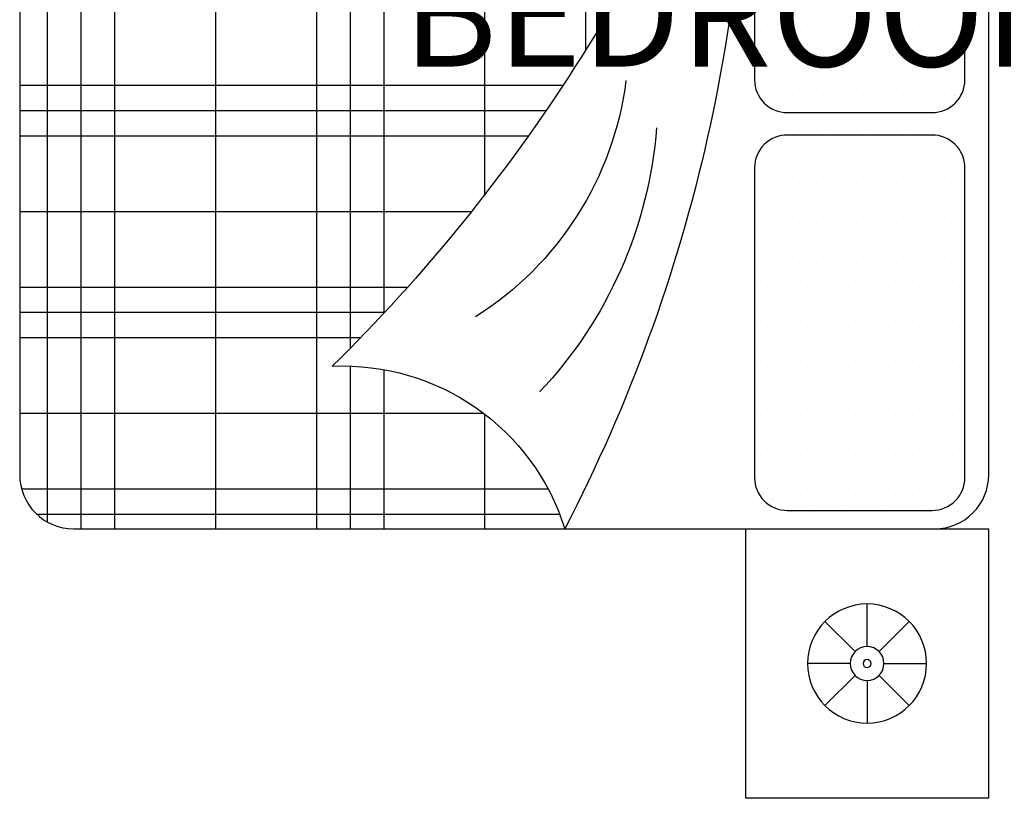
# Model space of a CAD drawing. Units: inches. Extents: x 528 to 2520, y -151 to 1354.
# Tile 23 of 41: x 1351 to 1407, y 1151 to 1195. Entities that reach past the tile are written whole.
import ezdxf

# ---------------------------------------------------------------- set-up
doc = ezdxf.new("R2010")
doc.units = ezdxf.units.IN
doc.header["$MEASUREMENT"] = 0
doc.layers.add('A-ANNO-DIMS', color=2, linetype='Continuous', lineweight=18)
doc.layers.add('A-FURN', color=8, linetype='Continuous', lineweight=18)
doc.layers.add('BLOCK', color=6, linetype='Continuous')
doc.styles.get("Standard").update_dxf_attribs({"font": 'arial.ttf'})
doc.dimstyles.get("Standard").update_dxf_attribs({"dimtxt": 6, "dimasz": 2, "dimexe": 0.18, "dimexo": 0.0625, "dimgap": 0.09, "dimtad": 0, "dimtih": 1, "dimtoh": 1, "dimdec": 1, "dimzin": 0, "dimdsep": 46, "dimlunit": 3, "dimtxsty": 'Standard', "dimblk": 'ARCHTICK', "dimcen": 0.09, "dimadec": 0, "dimazin": 0, "dimtfac": 1, "dimtdec": 1, "dimtofl": 0, "dimtmove": 0, "dimatfit": 3, "dimfxl": 1, "dimtolj": 1, "dimtzin": 0, "dimarcsym": 0})

# ---------------------------------------------------------------- blocks, each defined once
blk = doc.blocks.new('*X15')
at = {"color": 0}
for p, q in [((276.598, 451.25), (280.51, 451.25)), ((275.455, 450.625), (280.51, 450.625)), ((274.411, 450), (280.51, 450)), ((265.51, 448.125), (267.634, 448.125)), ((271.723, 448.125), (280.51, 448.125)), ((265.51, 446.25), (268.465, 446.25)), ((269.519, 446.25), (280.51, 446.25)), ((265.51, 445.625), (268.531, 445.625)), ((268.866, 445.625), (280.51, 445.625)), ((265.51, 445), (280.51, 445)), ((265.51, 443.125), (280.51, 443.125)), ((265.51, 441.25), (280.51, 441.25)), ((265.51, 440.625), (280.51, 440.625)), ((265.634, 440), (280.386, 440))]:
    blk.add_line(p, q, dxfattribs=at)
blk = doc.blocks.new('*X16')
at = {"color": 0}
for p, q in [((280.312, 439.886), (280.312, 452.896)), ((278.906, 439.482), (278.906, 452.338)), ((277.5, 439.482), (277.5, 451.702)), ((277.031, 439.482), (277.031, 451.471)), ((276.562, 439.482), (276.562, 451.231)), ((275.156, 439.482), (275.156, 450.451)), ((273.75, 439.482), (273.75, 449.576)), ((265.781, 439.797), (265.781, 449.511)), ((266.25, 439.517), (266.25, 449.296)), ((273.281, 439.482), (273.281, 449.261)), ((272.812, 439.482), (272.812, 448.934)), ((267.656, 439.482), (267.656, 448.095)), ((271.406, 439.482), (271.406, 447.876)), ((270, 439.482), (270, 446.689)), ((269.531, 439.482), (269.531, 446.262)), ((269.062, 439.482), (269.062, 445.817))]:
    blk.add_line(p, q, dxfattribs=at)
blk = doc.blocks.new('*X17')
at = {"color": 0}
for p, q in [((266.25, 456.9375), (266.25, 456.9375)), ((266.4375, 457.03125), (266.4375, 457.03125)), ((266.625, 456.9375), (266.625, 456.9375)), ((266.8125, 457.03125), (266.8125, 457.03125)), ((267, 456.9375), (267, 456.9375)), ((267.1875, 457.03125), (267.1875, 457.03125)), ((267.375, 456.9375), (267.375, 456.9375)), ((267.5625, 457.03125), (267.5625, 457.03125)), ((267.75, 456.9375), (267.75, 456.9375)), ((267.9375, 457.03125), (267.9375, 457.03125)), ((268.125, 456.9375), (268.125, 456.9375)), ((268.3125, 457.03125), (268.3125, 457.03125)), ((268.5, 456.9375), (268.5, 456.9375)), ((268.6875, 457.03125), (268.6875, 457.03125)), ((268.875, 456.9375), (268.875, 456.9375)), ((269.0625, 457.03125), (269.0625, 457.03125)), ((269.25, 456.9375), (269.25, 456.9375)), ((269.4375, 457.03125), (269.4375, 457.03125)), ((269.625, 456.9375), (269.625, 456.9375)), ((269.8125, 457.03125), (269.8125, 457.03125)), ((270, 456.9375), (270, 456.9375)), ((270.1875, 457.03125), (270.1875, 457.03125)), ((270.375, 456.9375), (270.375, 456.9375)), ((270.5625, 457.03125), (270.5625, 457.03125)), ((270.75, 456.9375), (270.75, 456.9375)), ((270.9375, 457.03125), (270.9375, 457.03125)), ((271.125, 456.9375), (271.125, 456.9375)), ((271.3125, 457.03125), (271.3125, 457.03125)), ((271.5, 456.9375), (271.5, 456.9375)), ((271.6875, 457.03125), (271.6875, 457.03125)), ((271.875, 456.9375), (271.875, 456.9375)), ((272.0625, 457.03125), (272.0625, 457.03125)), ((272.25, 456.9375), (272.25, 456.9375)), ((273.75, 456.9375), (273.75, 456.9375)), ((273.9375, 457.03125), (273.9375, 457.03125)), ((274.125, 456.9375), (274.125, 456.9375)), ((274.3125, 457.03125), (274.3125, 457.03125)), ((274.5, 456.9375), (274.5, 456.9375)), ((274.6875, 457.03125), (274.6875, 457.03125)), ((274.875, 456.9375), (274.875, 456.9375)), ((266.0625, 456.84375), (266.0625, 456.84375)), ((266.25, 456.75), (266.25, 456.75)), ((266.4375, 456.84375), (266.4375, 456.84375)), ((266.625, 456.75), (266.625, 456.75)), ((266.8125, 456.84375), (266.8125, 456.84375)), ((267, 456.75), (267, 456.75)), ((267.1875, 456.84375), (267.1875, 456.84375)), ((267.375, 456.75), (267.375, 456.75)), ((267.5625, 456.84375), (267.5625, 456.84375)), ((267.75, 456.75), (267.75, 456.75)), ((267.9375, 456.84375), (267.9375, 456.84375)), ((268.125, 456.75), (268.125, 456.75)), ((268.3125, 456.84375), (268.3125, 456.84375)), ((268.5, 456.75), (268.5, 456.75)), ((268.6875, 456.84375), (268.6875, 456.84375)), ((268.875, 456.75), (268.875, 456.75)), ((269.0625, 456.84375), (269.0625, 456.84375)), ((269.25, 456.75), (269.25, 456.75)), ((269.4375, 456.84375), (269.4375, 456.84375)), ((269.625, 456.75), (269.625, 456.75)), ((269.8125, 456.84375), (269.8125, 456.84375)), ((270, 456.75), (270, 456.75)), ((270.1875, 456.84375), (270.1875, 456.84375)), ((270.375, 456.75), (270.375, 456.75)), ((270.5625, 456.84375), (270.5625, 456.84375)), ((270.75, 456.75), (270.75, 456.75)), ((270.9375, 456.84375), (270.9375, 456.84375)), ((271.125, 456.75), (271.125, 456.75)), ((271.3125, 456.84375), (271.3125, 456.84375)), ((271.5, 456.75), (271.5, 456.75)), ((271.6875, 456.84375), (271.6875, 456.84375)), ((271.875, 456.75), (271.875, 456.75)), ((272.0625, 456.84375), (272.0625, 456.84375)), ((272.25, 456.75), (272.25, 456.75)), ((272.4375, 456.84375), (272.4375, 456.84375)), ((272.625, 456.75), (272.625, 456.75)), ((273.375, 456.75), (273.375, 456.75)), ((273.5625, 456.84375), (273.5625, 456.84375)), ((273.75, 456.75), (273.75, 456.75)), ((273.9375, 456.84375), (273.9375, 456.84375)), ((274.125, 456.75), (274.125, 456.75)), ((274.3125, 456.84375), (274.3125, 456.84375)), ((274.5, 456.75), (274.5, 456.75)), ((274.6875, 456.84375), (274.6875, 456.84375)), ((274.875, 456.75), (274.875, 456.75)), ((265.875, 456.5625), (265.875, 456.5625)), ((266.0625, 456.65625), (266.0625, 456.65625)), ((266.25, 456.5625), (266.25, 456.5625)), ((266.4375, 456.65625), (266.4375, 456.65625)), ((266.625, 456.5625), (266.625, 456.5625)), ((266.8125, 456.65625), (266.8125, 456.65625)), ((267, 456.5625), (267, 456.5625)), ((267.1875, 456.65625), (267.1875, 456.65625)), ((267.375, 456.5625), (267.375, 456.5625)), ((267.5625, 456.65625), (267.5625, 456.65625)), ((267.75, 456.5625), (267.75, 456.5625)), ((267.9375, 456.65625), (267.9375, 456.65625)), ((268.125, 456.5625), (268.125, 456.5625)), ((268.3125, 456.65625), (268.3125, 456.65625)), ((268.5, 456.5625), (268.5, 456.5625)), ((268.6875, 456.65625), (268.6875, 456.65625)), ((268.875, 456.5625), (268.875, 456.5625)), ((269.0625, 456.65625), (269.0625, 456.65625)), ((269.25, 456.5625), (269.25, 456.5625)), ((269.4375, 456.65625), (269.4375, 456.65625)), ((269.625, 456.5625), (269.625, 456.5625)), ((269.8125, 456.65625), (269.8125, 456.65625)), ((270, 456.5625), (270, 456.5625)), ((270.1875, 456.65625), (270.1875, 456.65625)), ((270.375, 456.5625), (270.375, 456.5625)), ((270.5625, 456.65625), (270.5625, 456.65625)), ((270.75, 456.5625), (270.75, 456.5625)), ((270.9375, 456.65625), (270.9375, 456.65625)), ((271.125, 456.5625), (271.125, 456.5625)), ((271.3125, 456.65625), (271.3125, 456.65625)), ((271.5, 456.5625), (271.5, 456.5625)), ((271.6875, 456.65625), (271.6875, 456.65625)), ((271.875, 456.5625), (271.875, 456.5625)), ((272.0625, 456.65625), (272.0625, 456.65625)), ((272.25, 456.5625), (272.25, 456.5625)), ((272.4375, 456.65625), (272.4375, 456.65625)), ((272.625, 456.5625), (272.625, 456.5625)), ((273.375, 456.5625), (273.375, 456.5625)), ((273.5625, 456.65625), (273.5625, 456.65625)), ((273.75, 456.5625), (273.75, 456.5625)), ((273.9375, 456.65625), (273.9375, 456.65625)), ((274.125, 456.5625), (274.125, 456.5625)), ((274.3125, 456.65625), (274.3125, 456.65625)), ((274.5, 456.5625), (274.5, 456.5625)), ((274.6875, 456.65625), (274.6875, 456.65625)), ((274.875, 456.5625), (274.875, 456.5625)), ((265.875, 456.375), (265.875, 456.375)), ((266.0625, 456.46875), (266.0625, 456.46875)), ((266.25, 456.375), (266.25, 456.375)), ((266.4375, 456.46875), (266.4375, 456.46875)), ((266.625, 456.375), (266.625, 456.375)), ((266.8125, 456.46875), (266.8125, 456.46875)), ((267, 456.375), (267, 456.375)), ((267.1875, 456.46875), (267.1875, 456.46875)), ((267.375, 456.375), (267.375, 456.375)), ((267.5625, 456.46875), (267.5625, 456.46875)), ((267.75, 456.375), (267.75, 456.375)), ((267.9375, 456.46875), (267.9375, 456.46875)), ((268.125, 456.375), (268.125, 456.375)), ((268.3125, 456.46875), (268.3125, 456.46875)), ((268.5, 456.375), (268.5, 456.375)), ((268.6875, 456.46875), (268.6875, 456.46875)), ((268.875, 456.375), (268.875, 456.375)), ((269.0625, 456.46875), (269.0625, 456.46875)), ((269.25, 456.375), (269.25, 456.375)), ((269.4375, 456.46875), (269.4375, 456.46875)), ((269.625, 456.375), (269.625, 456.375)), ((269.8125, 456.46875), (269.8125, 456.46875)), ((270, 456.375), (270, 456.375)), ((270.1875, 456.46875), (270.1875, 456.46875)), ((270.375, 456.375), (270.375, 456.375)), ((270.5625, 456.46875), (270.5625, 456.46875)), ((270.75, 456.375), (270.75, 456.375)), ((270.9375, 456.46875), (270.9375, 456.46875)), ((271.125, 456.375), (271.125, 456.375)), ((271.3125, 456.46875), (271.3125, 456.46875)), ((271.5, 456.375), (271.5, 456.375)), ((271.6875, 456.46875), (271.6875, 456.46875)), ((271.875, 456.375), (271.875, 456.375)), ((272.0625, 456.46875), (272.0625, 456.46875)), ((272.25, 456.375), (272.25, 456.375)), ((272.4375, 456.46875), (272.4375, 456.46875)), ((272.625, 456.375), (272.625, 456.375)), ((272.8125, 456.46875), (272.8125, 456.46875)), ((273.375, 456.375), (273.375, 456.375)), ((273.5625, 456.46875), (273.5625, 456.46875)), ((273.75, 456.375), (273.75, 456.375)), ((273.9375, 456.46875), (273.9375, 456.46875)), ((274.125, 456.375), (274.125, 456.375)), ((274.3125, 456.46875), (274.3125, 456.46875)), ((274.5, 456.375), (274.5, 456.375)), ((274.6875, 456.46875), (274.6875, 456.46875)), ((274.875, 456.375), (274.875, 456.375)), ((265.875, 456.1875), (265.875, 456.1875)), ((266.0625, 456.28125), (266.0625, 456.28125)), ((266.25, 456.1875), (266.25, 456.1875)), ((266.4375, 456.28125), (266.4375, 456.28125)), ((266.625, 456.1875), (266.625, 456.1875)), ((266.8125, 456.28125), (266.8125, 456.28125)), ((267, 456.1875), (267, 456.1875)), ((267.1875, 456.28125), (267.1875, 456.28125)), ((267.375, 456.1875), (267.375, 456.1875)), ((267.5625, 456.28125), (267.5625, 456.28125)), ((267.75, 456.1875), (267.75, 456.1875)), ((267.9375, 456.28125), (267.9375, 456.28125)), ((268.125, 456.1875), (268.125, 456.1875)), ((268.3125, 456.28125), (268.3125, 456.28125)), ((268.5, 456.1875), (268.5, 456.1875)), ((268.6875, 456.28125), (268.6875, 456.28125)), ((268.875, 456.1875), (268.875, 456.1875)), ((269.0625, 456.28125), (269.0625, 456.28125)), ((269.25, 456.1875), (269.25, 456.1875)), ((269.4375, 456.28125), (269.4375, 456.28125)), ((269.625, 456.1875), (269.625, 456.1875)), ((269.8125, 456.28125), (269.8125, 456.28125)), ((270, 456.1875), (270, 456.1875)), ((270.1875, 456.28125), (270.1875, 456.28125)), ((270.375, 456.1875), (270.375, 456.1875)), ((270.5625, 456.28125), (270.5625, 456.28125)), ((270.75, 456.1875), (270.75, 456.1875)), ((270.9375, 456.28125), (270.9375, 456.28125)), ((271.125, 456.1875), (271.125, 456.1875)), ((271.3125, 456.28125), (271.3125, 456.28125)), ((271.5, 456.1875), (271.5, 456.1875)), ((271.6875, 456.28125), (271.6875, 456.28125)), ((271.875, 456.1875), (271.875, 456.1875)), ((272.0625, 456.28125), (272.0625, 456.28125)), ((272.25, 456.1875), (272.25, 456.1875)), ((272.4375, 456.28125), (272.4375, 456.28125)), ((272.625, 456.1875), (272.625, 456.1875)), ((272.8125, 456.28125), (272.8125, 456.28125)), ((273.375, 456.1875), (273.375, 456.1875)), ((273.5625, 456.28125), (273.5625, 456.28125)), ((273.75, 456.1875), (273.75, 456.1875)), ((273.9375, 456.28125), (273.9375, 456.28125)), ((274.125, 456.1875), (274.125, 456.1875)), ((274.3125, 456.28125), (274.3125, 456.28125)), ((274.5, 456.1875), (274.5, 456.1875)), ((274.6875, 456.28125), (274.6875, 456.28125)), ((274.875, 456.1875), (274.875, 456.1875)), ((265.875, 456), (265.875, 456)), ((266.0625, 456.09375), (266.0625, 456.09375)), ((266.25, 456), (266.25, 456)), ((266.4375, 456.09375), (266.4375, 456.09375)), ((266.625, 456), (266.625, 456)), ((266.8125, 456.09375), (266.8125, 456.09375)), ((267, 456), (267, 456)), ((267.1875, 456.09375), (267.1875, 456.09375)), ((267.375, 456), (267.375, 456)), ((267.5625, 456.09375), (267.5625, 456.09375)), ((267.75, 456), (267.75, 456)), ((267.9375, 456.09375), (267.9375, 456.09375)), ((268.125, 456), (268.125, 456)), ((268.3125, 456.09375), (268.3125, 456.09375)), ((268.5, 456), (268.5, 456)), ((268.6875, 456.09375), (268.6875, 456.09375)), ((268.875, 456), (268.875, 456)), ((269.0625, 456.09375), (269.0625, 456.09375)), ((269.25, 456), (269.25, 456)), ((269.4375, 456.09375), (269.4375, 456.09375)), ((269.625, 456), (269.625, 456)), ((269.8125, 456.09375), (269.8125, 456.09375)), ((270, 456), (270, 456)), ((270.1875, 456.09375), (270.1875, 456.09375)), ((270.375, 456), (270.375, 456)), ((270.5625, 456.09375), (270.5625, 456.09375)), ((270.75, 456), (270.75, 456)), ((270.9375, 456.09375), (270.9375, 456.09375)), ((271.125, 456), (271.125, 456)), ((271.3125, 456.09375), (271.3125, 456.09375)), ((271.5, 456), (271.5, 456)), ((271.6875, 456.09375), (271.6875, 456.09375)), ((271.875, 456), (271.875, 456)), ((272.0625, 456.09375), (272.0625, 456.09375)), ((272.25, 456), (272.25, 456)), ((272.4375, 456.09375), (272.4375, 456.09375)), ((272.625, 456), (272.625, 456)), ((272.8125, 456.09375), (272.8125, 456.09375)), ((273.375, 456), (273.375, 456)), ((273.5625, 456.09375), (273.5625, 456.09375)), ((273.75, 456), (273.75, 456)), ((273.9375, 456.09375), (273.9375, 456.09375)), ((274.125, 456), (274.125, 456)), ((274.3125, 456.09375), (274.3125, 456.09375)), ((274.5, 456), (274.5, 456)), ((274.6875, 456.09375), (274.6875, 456.09375)), ((274.875, 456), (274.875, 456)), ((265.875, 455.8125), (265.875, 455.8125)), ((266.0625, 455.90625), (266.0625, 455.90625)), ((266.25, 455.8125), (266.25, 455.8125)), ((266.4375, 455.90625), (266.4375, 455.90625)), ((266.625, 455.8125), (266.625, 455.8125)), ((266.8125, 455.90625), (266.8125, 455.90625)), ((267, 455.8125), (267, 455.8125)), ((267.1875, 455.90625), (267.1875, 455.90625)), ((267.375, 455.8125), (267.375, 455.8125)), ((267.5625, 455.90625), (267.5625, 455.90625)), ((267.75, 455.8125), (267.75, 455.8125)), ((267.9375, 455.90625), (267.9375, 455.90625)), ((268.125, 455.8125), (268.125, 455.8125)), ((268.3125, 455.90625), (268.3125, 455.90625)), ((268.5, 455.8125), (268.5, 455.8125)), ((268.6875, 455.90625), (268.6875, 455.90625)), ((268.875, 455.8125), (268.875, 455.8125)), ((269.0625, 455.90625), (269.0625, 455.90625)), ((269.25, 455.8125), (269.25, 455.8125)), ((269.4375, 455.90625), (269.4375, 455.90625)), ((269.625, 455.8125), (269.625, 455.8125)), ((269.8125, 455.90625), (269.8125, 455.90625)), ((270, 455.8125), (270, 455.8125)), ((270.1875, 455.90625), (270.1875, 455.90625)), ((270.375, 455.8125), (270.375, 455.8125)), ((270.5625, 455.90625), (270.5625, 455.90625)), ((270.75, 455.8125), (270.75, 455.8125)), ((270.9375, 455.90625), (270.9375, 455.90625)), ((271.125, 455.8125), (271.125, 455.8125)), ((271.3125, 455.90625), (271.3125, 455.90625)), ((271.5, 455.8125), (271.5, 455.8125)), ((271.6875, 455.90625), (271.6875, 455.90625)), ((271.875, 455.8125), (271.875, 455.8125)), ((272.0625, 455.90625), (272.0625, 455.90625)), ((272.25, 455.8125), (272.25, 455.8125)), ((272.4375, 455.90625), (272.4375, 455.90625)), ((272.625, 455.8125), (272.625, 455.8125)), ((272.8125, 455.90625), (272.8125, 455.90625)), ((273.375, 455.8125), (273.375, 455.8125)), ((273.5625, 455.90625), (273.5625, 455.90625)), ((273.75, 455.8125), (273.75, 455.8125)), ((273.9375, 455.90625), (273.9375, 455.90625)), ((274.125, 455.8125), (274.125, 455.8125)), ((274.3125, 455.90625), (274.3125, 455.90625)), ((274.5, 455.8125), (274.5, 455.8125)), ((274.6875, 455.90625), (274.6875, 455.90625)), ((274.875, 455.8125), (274.875, 455.8125)), ((265.875, 455.625), (265.875, 455.625)), ((266.0625, 455.71875), (266.0625, 455.71875)), ((266.25, 455.625), (266.25, 455.625)), ((266.4375, 455.71875), (266.4375, 455.71875)), ((266.625, 455.625), (266.625, 455.625)), ((266.8125, 455.71875), (266.8125, 455.71875)), ((267, 455.625), (267, 455.625)), ((267.1875, 455.71875), (267.1875, 455.71875)), ((267.375, 455.625), (267.375, 455.625)), ((267.5625, 455.71875), (267.5625, 455.71875)), ((267.75, 455.625), (267.75, 455.625)), ((267.9375, 455.71875), (267.9375, 455.71875)), ((268.125, 455.625), (268.125, 455.625)), ((268.3125, 455.71875), (268.3125, 455.71875)), ((268.5, 455.625), (268.5, 455.625)), ((268.6875, 455.71875), (268.6875, 455.71875)), ((268.875, 455.625), (268.875, 455.625)), ((269.0625, 455.71875), (269.0625, 455.71875)), ((269.25, 455.625), (269.25, 455.625)), ((269.4375, 455.71875), (269.4375, 455.71875)), ((269.625, 455.625), (269.625, 455.625)), ((269.8125, 455.71875), (269.8125, 455.71875)), ((270, 455.625), (270, 455.625)), ((270.1875, 455.71875), (270.1875, 455.71875)), ((270.375, 455.625), (270.375, 455.625)), ((270.5625, 455.71875), (270.5625, 455.71875)), ((270.75, 455.625), (270.75, 455.625)), ((270.9375, 455.71875), (270.9375, 455.71875)), ((271.125, 455.625), (271.125, 455.625)), ((271.3125, 455.71875), (271.3125, 455.71875)), ((271.5, 455.625), (271.5, 455.625)), ((271.6875, 455.71875), (271.6875, 455.71875)), ((271.875, 455.625), (271.875, 455.625)), ((272.0625, 455.71875), (272.0625, 455.71875)), ((272.25, 455.625), (272.25, 455.625)), ((272.4375, 455.71875), (272.4375, 455.71875)), ((272.625, 455.625), (272.625, 455.625)), ((272.8125, 455.71875), (272.8125, 455.71875)), ((273.375, 455.625), (273.375, 455.625)), ((273.5625, 455.71875), (273.5625, 455.71875)), ((273.75, 455.625), (273.75, 455.625)), ((273.9375, 455.71875), (273.9375, 455.71875)), ((274.125, 455.625), (274.125, 455.625)), ((274.3125, 455.71875), (274.3125, 455.71875)), ((274.5, 455.625), (274.5, 455.625)), ((274.6875, 455.71875), (274.6875, 455.71875)), ((274.875, 455.625), (274.875, 455.625)), ((265.875, 455.4375), (265.875, 455.4375)), ((266.0625, 455.53125), (266.0625, 455.53125)), ((266.25, 455.4375), (266.25, 455.4375)), ((266.4375, 455.53125), (266.4375, 455.53125)), ((266.625, 455.4375), (266.625, 455.4375)), ((266.8125, 455.53125), (266.8125, 455.53125)), ((267, 455.4375), (267, 455.4375)), ((267.1875, 455.53125), (267.1875, 455.53125)), ((267.375, 455.4375), (267.375, 455.4375)), ((267.5625, 455.53125), (267.5625, 455.53125)), ((267.75, 455.4375), (267.75, 455.4375)), ((267.9375, 455.53125), (267.9375, 455.53125)), ((268.125, 455.4375), (268.125, 455.4375)), ((268.3125, 455.53125), (268.3125, 455.53125)), ((268.5, 455.4375), (268.5, 455.4375)), ((268.6875, 455.53125), (268.6875, 455.53125)), ((268.875, 455.4375), (268.875, 455.4375)), ((269.0625, 455.53125), (269.0625, 455.53125)), ((269.25, 455.4375), (269.25, 455.4375)), ((269.4375, 455.53125), (269.4375, 455.53125)), ((269.625, 455.4375), (269.625, 455.4375)), ((269.8125, 455.53125), (269.8125, 455.53125)), ((270, 455.4375), (270, 455.4375)), ((270.1875, 455.53125), (270.1875, 455.53125)), ((270.375, 455.4375), (270.375, 455.4375)), ((270.5625, 455.53125), (270.5625, 455.53125)), ((270.75, 455.4375), (270.75, 455.4375)), ((270.9375, 455.53125), (270.9375, 455.53125)), ((271.125, 455.4375), (271.125, 455.4375)), ((271.3125, 455.53125), (271.3125, 455.53125)), ((271.5, 455.4375), (271.5, 455.4375)), ((271.6875, 455.53125), (271.6875, 455.53125)), ((271.875, 455.4375), (271.875, 455.4375)), ((272.0625, 455.53125), (272.0625, 455.53125)), ((272.25, 455.4375), (272.25, 455.4375)), ((272.4375, 455.53125), (272.4375, 455.53125)), ((272.625, 455.4375), (272.625, 455.4375)), ((272.8125, 455.53125), (272.8125, 455.53125)), ((273.375, 455.4375), (273.375, 455.4375)), ((273.5625, 455.53125), (273.5625, 455.53125)), ((273.75, 455.4375), (273.75, 455.4375)), ((273.9375, 455.53125), (273.9375, 455.53125)), ((274.125, 455.4375), (274.125, 455.4375)), ((274.3125, 455.53125), (274.3125, 455.53125)), ((274.5, 455.4375), (274.5, 455.4375)), ((274.6875, 455.53125), (274.6875, 455.53125)), ((274.875, 455.4375), (274.875, 455.4375)), ((265.875, 455.25), (265.875, 455.25)), ((266.0625, 455.34375), (266.0625, 455.34375)), ((266.25, 455.25), (266.25, 455.25)), ((266.4375, 455.34375), (266.4375, 455.34375)), ((266.625, 455.25), (266.625, 455.25)), ((266.8125, 455.34375), (266.8125, 455.34375)), ((267, 455.25), (267, 455.25)), ((267.1875, 455.34375), (267.1875, 455.34375)), ((267.375, 455.25), (267.375, 455.25)), ((267.5625, 455.34375), (267.5625, 455.34375)), ((267.75, 455.25), (267.75, 455.25)), ((267.9375, 455.34375), (267.9375, 455.34375)), ((268.125, 455.25), (268.125, 455.25)), ((268.3125, 455.34375), (268.3125, 455.34375)), ((268.5, 455.25), (268.5, 455.25)), ((268.6875, 455.34375), (268.6875, 455.34375)), ((268.875, 455.25), (268.875, 455.25)), ((269.0625, 455.34375), (269.0625, 455.34375)), ((269.25, 455.25), (269.25, 455.25)), ((269.4375, 455.34375), (269.4375, 455.34375)), ((269.625, 455.25), (269.625, 455.25)), ((269.8125, 455.34375), (269.8125, 455.34375)), ((270, 455.25), (270, 455.25)), ((270.1875, 455.34375), (270.1875, 455.34375)), ((270.375, 455.25), (270.375, 455.25)), ((270.5625, 455.34375), (270.5625, 455.34375)), ((270.75, 455.25), (270.75, 455.25)), ((270.9375, 455.34375), (270.9375, 455.34375)), ((271.125, 455.25), (271.125, 455.25)), ((271.3125, 455.34375), (271.3125, 455.34375)), ((271.5, 455.25), (271.5, 455.25)), ((271.6875, 455.34375), (271.6875, 455.34375)), ((271.875, 455.25), (271.875, 455.25)), ((272.0625, 455.34375), (272.0625, 455.34375)), ((272.25, 455.25), (272.25, 455.25)), ((272.4375, 455.34375), (272.4375, 455.34375)), ((272.625, 455.25), (272.625, 455.25)), ((272.8125, 455.34375), (272.8125, 455.34375)), ((273.375, 455.25), (273.375, 455.25)), ((273.5625, 455.34375), (273.5625, 455.34375)), ((273.75, 455.25), (273.75, 455.25)), ((273.9375, 455.34375), (273.9375, 455.34375)), ((274.125, 455.25), (274.125, 455.25)), ((274.3125, 455.34375), (274.3125, 455.34375)), ((274.5, 455.25), (274.5, 455.25)), ((274.6875, 455.34375), (274.6875, 455.34375)), ((274.875, 455.25), (274.875, 455.25)), ((265.875, 455.0625), (265.875, 455.0625)), ((266.0625, 455.15625), (266.0625, 455.15625)), ((266.25, 455.0625), (266.25, 455.0625)), ((266.4375, 455.15625), (266.4375, 455.15625)), ((266.625, 455.0625), (266.625, 455.0625)), ((266.8125, 455.15625), (266.8125, 455.15625)), ((267, 455.0625), (267, 455.0625)), ((267.1875, 455.15625), (267.1875, 455.15625)), ((267.375, 455.0625), (267.375, 455.0625)), ((267.5625, 455.15625), (267.5625, 455.15625)), ((267.75, 455.0625), (267.75, 455.0625)), ((267.9375, 455.15625), (267.9375, 455.15625)), ((268.125, 455.0625), (268.125, 455.0625)), ((268.3125, 455.15625), (268.3125, 455.15625)), ((268.5, 455.0625), (268.5, 455.0625)), ((268.6875, 455.15625), (268.6875, 455.15625)), ((268.875, 455.0625), (268.875, 455.0625)), ((269.0625, 455.15625), (269.0625, 455.15625)), ((269.25, 455.0625), (269.25, 455.0625)), ((269.4375, 455.15625), (269.4375, 455.15625)), ((269.625, 455.0625), (269.625, 455.0625)), ((269.8125, 455.15625), (269.8125, 455.15625)), ((270, 455.0625), (270, 455.0625)), ((270.1875, 455.15625), (270.1875, 455.15625)), ((270.375, 455.0625), (270.375, 455.0625)), ((270.5625, 455.15625), (270.5625, 455.15625)), ((270.75, 455.0625), (270.75, 455.0625)), ((270.9375, 455.15625), (270.9375, 455.15625)), ((271.125, 455.0625), (271.125, 455.0625)), ((271.3125, 455.15625), (271.3125, 455.15625)), ((271.5, 455.0625), (271.5, 455.0625)), ((271.6875, 455.15625), (271.6875, 455.15625)), ((271.875, 455.0625), (271.875, 455.0625)), ((272.0625, 455.15625), (272.0625, 455.15625)), ((272.25, 455.0625), (272.25, 455.0625)), ((272.4375, 455.15625), (272.4375, 455.15625)), ((272.625, 455.0625), (272.625, 455.0625)), ((272.8125, 455.15625), (272.8125, 455.15625)), ((273.375, 455.0625), (273.375, 455.0625)), ((273.5625, 455.15625), (273.5625, 455.15625)), ((273.75, 455.0625), (273.75, 455.0625)), ((273.9375, 455.15625), (273.9375, 455.15625)), ((274.125, 455.0625), (274.125, 455.0625)), ((274.3125, 455.15625), (274.3125, 455.15625)), ((274.5, 455.0625), (274.5, 455.0625)), ((274.6875, 455.15625), (274.6875, 455.15625)), ((274.875, 455.0625), (274.875, 455.0625)), ((265.875, 454.875), (265.875, 454.875)), ((266.0625, 454.96875), (266.0625, 454.96875)), ((266.25, 454.875), (266.25, 454.875)), ((266.4375, 454.96875), (266.4375, 454.96875)), ((266.625, 454.875), (266.625, 454.875)), ((266.8125, 454.96875), (266.8125, 454.96875)), ((267, 454.875), (267, 454.875)), ((267.1875, 454.96875), (267.1875, 454.96875)), ((267.375, 454.875), (267.375, 454.875)), ((267.5625, 454.96875), (267.5625, 454.96875)), ((267.75, 454.875), (267.75, 454.875)), ((267.9375, 454.96875), (267.9375, 454.96875)), ((268.125, 454.875), (268.125, 454.875)), ((268.3125, 454.96875), (268.3125, 454.96875)), ((268.5, 454.875), (268.5, 454.875)), ((268.6875, 454.96875), (268.6875, 454.96875)), ((268.875, 454.875), (268.875, 454.875)), ((269.0625, 454.96875), (269.0625, 454.96875)), ((269.25, 454.875), (269.25, 454.875)), ((269.4375, 454.96875), (269.4375, 454.96875)), ((269.625, 454.875), (269.625, 454.875)), ((269.8125, 454.96875), (269.8125, 454.96875)), ((270, 454.875), (270, 454.875)), ((270.1875, 454.96875), (270.1875, 454.96875)), ((270.375, 454.875), (270.375, 454.875)), ((270.5625, 454.96875), (270.5625, 454.96875)), ((270.75, 454.875), (270.75, 454.875)), ((270.9375, 454.96875), (270.9375, 454.96875)), ((271.125, 454.875), (271.125, 454.875)), ((271.3125, 454.96875), (271.3125, 454.96875)), ((271.5, 454.875), (271.5, 454.875)), ((271.6875, 454.96875), (271.6875, 454.96875)), ((271.875, 454.875), (271.875, 454.875)), ((272.0625, 454.96875), (272.0625, 454.96875)), ((272.25, 454.875), (272.25, 454.875)), ((272.4375, 454.96875), (272.4375, 454.96875)), ((272.625, 454.875), (272.625, 454.875)), ((272.8125, 454.96875), (272.8125, 454.96875)), ((273.375, 454.875), (273.375, 454.875)), ((273.5625, 454.96875), (273.5625, 454.96875)), ((273.75, 454.875), (273.75, 454.875)), ((273.9375, 454.96875), (273.9375, 454.96875)), ((274.125, 454.875), (274.125, 454.875)), ((274.3125, 454.96875), (274.3125, 454.96875)), ((274.5, 454.875), (274.5, 454.875)), ((274.6875, 454.96875), (274.6875, 454.96875)), ((274.875, 454.875), (274.875, 454.875)), ((265.875, 454.6875), (265.875, 454.6875)), ((266.0625, 454.78125), (266.0625, 454.78125)), ((266.25, 454.6875), (266.25, 454.6875)), ((266.4375, 454.78125), (266.4375, 454.78125)), ((266.625, 454.6875), (266.625, 454.6875)), ((266.8125, 454.78125), (266.8125, 454.78125)), ((267, 454.6875), (267, 454.6875)), ((267.1875, 454.78125), (267.1875, 454.78125)), ((267.375, 454.6875), (267.375, 454.6875)), ((267.5625, 454.78125), (267.5625, 454.78125)), ((267.75, 454.6875), (267.75, 454.6875)), ((267.9375, 454.78125), (267.9375, 454.78125)), ((268.125, 454.6875), (268.125, 454.6875)), ((268.3125, 454.78125), (268.3125, 454.78125)), ((268.5, 454.6875), (268.5, 454.6875)), ((268.6875, 454.78125), (268.6875, 454.78125)), ((268.875, 454.6875), (268.875, 454.6875)), ((269.0625, 454.78125), (269.0625, 454.78125)), ((269.25, 454.6875), (269.25, 454.6875)), ((269.4375, 454.78125), (269.4375, 454.78125)), ((269.625, 454.6875), (269.625, 454.6875)), ((269.8125, 454.78125), (269.8125, 454.78125)), ((270, 454.6875), (270, 454.6875)), ((270.1875, 454.78125), (270.1875, 454.78125)), ((270.375, 454.6875), (270.375, 454.6875)), ((270.5625, 454.78125), (270.5625, 454.78125)), ((270.75, 454.6875), (270.75, 454.6875)), ((270.9375, 454.78125), (270.9375, 454.78125)), ((271.125, 454.6875), (271.125, 454.6875)), ((271.3125, 454.78125), (271.3125, 454.78125)), ((271.5, 454.6875), (271.5, 454.6875)), ((271.6875, 454.78125), (271.6875, 454.78125)), ((271.875, 454.6875), (271.875, 454.6875)), ((272.0625, 454.78125), (272.0625, 454.78125)), ((272.25, 454.6875), (272.25, 454.6875)), ((272.4375, 454.78125), (272.4375, 454.78125)), ((272.625, 454.6875), (272.625, 454.6875)), ((272.8125, 454.78125), (272.8125, 454.78125)), ((273.375, 454.6875), (273.375, 454.6875)), ((273.5625, 454.78125), (273.5625, 454.78125)), ((273.75, 454.6875), (273.75, 454.6875)), ((273.9375, 454.78125), (273.9375, 454.78125)), ((274.125, 454.6875), (274.125, 454.6875)), ((274.3125, 454.78125), (274.3125, 454.78125)), ((274.5, 454.6875), (274.5, 454.6875)), ((274.6875, 454.78125), (274.6875, 454.78125)), ((274.875, 454.6875), (274.875, 454.6875)), ((266.0625, 454.59375), (266.0625, 454.59375)), ((266.4375, 454.59375), (266.4375, 454.59375)), ((266.8125, 454.59375), (266.8125, 454.59375)), ((267.1875, 454.59375), (267.1875, 454.59375)), ((267.5625, 454.59375), (267.5625, 454.59375)), ((267.9375, 454.59375), (267.9375, 454.59375)), ((268.3125, 454.59375), (268.3125, 454.59375)), ((268.6875, 454.59375), (268.6875, 454.59375)), ((269.0625, 454.59375), (269.0625, 454.59375)), ((269.4375, 454.59375), (269.4375, 454.59375)), ((269.8125, 454.59375), (269.8125, 454.59375)), ((270.1875, 454.59375), (270.1875, 454.59375)), ((270.5625, 454.59375), (270.5625, 454.59375)), ((270.9375, 454.59375), (270.9375, 454.59375)), ((271.3125, 454.59375), (271.3125, 454.59375)), ((271.6875, 454.59375), (271.6875, 454.59375)), ((272.0625, 454.59375), (272.0625, 454.59375)), ((272.4375, 454.59375), (272.4375, 454.59375)), ((272.8125, 454.59375), (272.8125, 454.59375)), ((273.5625, 454.59375), (273.5625, 454.59375)), ((273.9375, 454.59375), (273.9375, 454.59375)), ((274.3125, 454.59375), (274.3125, 454.59375)), ((274.6875, 454.59375), (274.6875, 454.59375)), ((265.875, 454.5), (265.875, 454.5)), ((266.0625, 454.40625), (266.0625, 454.40625)), ((266.25, 454.5), (266.25, 454.5)), ((266.4375, 454.40625), (266.4375, 454.40625)), ((266.625, 454.5), (266.625, 454.5)), ((266.8125, 454.40625), (266.8125, 454.40625)), ((267, 454.5), (267, 454.5)), ((267.1875, 454.40625), (267.1875, 454.40625)), ((267.375, 454.5), (267.375, 454.5)), ((267.5625, 454.40625), (267.5625, 454.40625)), ((267.75, 454.5), (267.75, 454.5)), ((267.9375, 454.40625), (267.9375, 454.40625)), ((268.125, 454.5), (268.125, 454.5)), ((268.3125, 454.40625), (268.3125, 454.40625)), ((268.5, 454.5), (268.5, 454.5)), ((268.6875, 454.40625), (268.6875, 454.40625)), ((268.875, 454.5), (268.875, 454.5)), ((269.0625, 454.40625), (269.0625, 454.40625)), ((269.25, 454.5), (269.25, 454.5)), ((269.4375, 454.40625), (269.4375, 454.40625)), ((269.625, 454.5), (269.625, 454.5)), ((269.8125, 454.40625), (269.8125, 454.40625)), ((270, 454.5), (270, 454.5)), ((270.1875, 454.40625), (270.1875, 454.40625)), ((270.375, 454.5), (270.375, 454.5)), ((270.5625, 454.40625), (270.5625, 454.40625)), ((270.75, 454.5), (270.75, 454.5)), ((270.9375, 454.40625), (270.9375, 454.40625)), ((271.125, 454.5), (271.125, 454.5)), ((271.3125, 454.40625), (271.3125, 454.40625)), ((271.5, 454.5), (271.5, 454.5)), ((271.6875, 454.40625), (271.6875, 454.40625)), ((271.875, 454.5), (271.875, 454.5)), ((272.0625, 454.40625), (272.0625, 454.40625)), ((272.25, 454.5), (272.25, 454.5)), ((272.4375, 454.40625), (272.4375, 454.40625)), ((272.625, 454.5), (272.625, 454.5)), ((272.8125, 454.40625), (272.8125, 454.40625)), ((273.375, 454.5), (273.375, 454.5)), ((273.5625, 454.40625), (273.5625, 454.40625)), ((273.75, 454.5), (273.75, 454.5)), ((273.9375, 454.40625), (273.9375, 454.40625)), ((274.125, 454.5), (274.125, 454.5)), ((274.3125, 454.40625), (274.3125, 454.40625)), ((274.5, 454.5), (274.5, 454.5)), ((274.6875, 454.40625), (274.6875, 454.40625)), ((274.875, 454.5), (274.875, 454.5)), ((265.875, 454.3125), (265.875, 454.3125)), ((266.0625, 454.21875), (266.0625, 454.21875)), ((266.25, 454.3125), (266.25, 454.3125)), ((266.4375, 454.21875), (266.4375, 454.21875)), ((266.625, 454.3125), (266.625, 454.3125)), ((266.8125, 454.21875), (266.8125, 454.21875)), ((267, 454.3125), (267, 454.3125)), ((267.1875, 454.21875), (267.1875, 454.21875)), ((267.375, 454.3125), (267.375, 454.3125)), ((267.5625, 454.21875), (267.5625, 454.21875)), ((267.75, 454.3125), (267.75, 454.3125)), ((267.9375, 454.21875), (267.9375, 454.21875)), ((268.125, 454.3125), (268.125, 454.3125)), ((268.3125, 454.21875), (268.3125, 454.21875)), ((268.5, 454.3125), (268.5, 454.3125)), ((268.6875, 454.21875), (268.6875, 454.21875)), ((268.875, 454.3125), (268.875, 454.3125)), ((269.0625, 454.21875), (269.0625, 454.21875)), ((269.25, 454.3125), (269.25, 454.3125)), ((269.4375, 454.21875), (269.4375, 454.21875)), ((269.625, 454.3125), (269.625, 454.3125)), ((269.8125, 454.21875), (269.8125, 454.21875)), ((270, 454.3125), (270, 454.3125)), ((270.1875, 454.21875), (270.1875, 454.21875)), ((270.375, 454.3125), (270.375, 454.3125)), ((270.5625, 454.21875), (270.5625, 454.21875)), ((270.75, 454.3125), (270.75, 454.3125)), ((270.9375, 454.21875), (270.9375, 454.21875)), ((271.125, 454.3125), (271.125, 454.3125)), ((271.3125, 454.21875), (271.3125, 454.21875)), ((271.5, 454.3125), (271.5, 454.3125)), ((271.6875, 454.21875), (271.6875, 454.21875)), ((271.875, 454.3125), (271.875, 454.3125)), ((272.0625, 454.21875), (272.0625, 454.21875)), ((272.25, 454.3125), (272.25, 454.3125)), ((272.4375, 454.21875), (272.4375, 454.21875)), ((272.625, 454.3125), (272.625, 454.3125)), ((272.8125, 454.21875), (272.8125, 454.21875)), ((273.375, 454.3125), (273.375, 454.3125)), ((273.5625, 454.21875), (273.5625, 454.21875)), ((273.75, 454.3125), (273.75, 454.3125)), ((273.9375, 454.21875), (273.9375, 454.21875)), ((274.125, 454.3125), (274.125, 454.3125)), ((274.3125, 454.21875), (274.3125, 454.21875)), ((274.5, 454.3125), (274.5, 454.3125)), ((274.6875, 454.21875), (274.6875, 454.21875)), ((274.875, 454.3125), (274.875, 454.3125)), ((265.875, 454.125), (265.875, 454.125)), ((266.0625, 454.03125), (266.0625, 454.03125)), ((266.25, 454.125), (266.25, 454.125)), ((266.4375, 454.03125), (266.4375, 454.03125)), ((266.625, 454.125), (266.625, 454.125)), ((266.8125, 454.03125), (266.8125, 454.03125)), ((267, 454.125), (267, 454.125)), ((267.1875, 454.03125), (267.1875, 454.03125)), ((267.375, 454.125), (267.375, 454.125)), ((267.5625, 454.03125), (267.5625, 454.03125)), ((267.75, 454.125), (267.75, 454.125)), ((267.9375, 454.03125), (267.9375, 454.03125)), ((268.125, 454.125), (268.125, 454.125)), ((268.3125, 454.03125), (268.3125, 454.03125)), ((268.5, 454.125), (268.5, 454.125)), ((268.6875, 454.03125), (268.6875, 454.03125)), ((268.875, 454.125), (268.875, 454.125)), ((269.0625, 454.03125), (269.0625, 454.03125)), ((269.25, 454.125), (269.25, 454.125)), ((269.4375, 454.03125), (269.4375, 454.03125)), ((269.625, 454.125), (269.625, 454.125)), ((269.8125, 454.03125), (269.8125, 454.03125)), ((270, 454.125), (270, 454.125)), ((270.1875, 454.03125), (270.1875, 454.03125)), ((270.375, 454.125), (270.375, 454.125)), ((270.5625, 454.03125), (270.5625, 454.03125)), ((270.75, 454.125), (270.75, 454.125)), ((270.9375, 454.03125), (270.9375, 454.03125)), ((271.125, 454.125), (271.125, 454.125)), ((271.3125, 454.03125), (271.3125, 454.03125)), ((271.5, 454.125), (271.5, 454.125)), ((271.6875, 454.03125), (271.6875, 454.03125)), ((271.875, 454.125), (271.875, 454.125)), ((272.0625, 454.03125), (272.0625, 454.03125)), ((272.25, 454.125), (272.25, 454.125)), ((272.4375, 454.03125), (272.4375, 454.03125)), ((272.625, 454.125), (272.625, 454.125)), ((272.8125, 454.03125), (272.8125, 454.03125)), ((273.375, 454.125), (273.375, 454.125)), ((273.5625, 454.03125), (273.5625, 454.03125)), ((273.75, 454.125), (273.75, 454.125)), ((273.9375, 454.03125), (273.9375, 454.03125)), ((274.125, 454.125), (274.125, 454.125)), ((274.3125, 454.03125), (274.3125, 454.03125)), ((274.5, 454.125), (274.5, 454.125)), ((274.6875, 454.03125), (274.6875, 454.03125)), ((274.875, 454.125), (274.875, 454.125)), ((265.875, 453.9375), (265.875, 453.9375)), ((266.0625, 453.84375), (266.0625, 453.84375)), ((266.25, 453.9375), (266.25, 453.9375)), ((266.4375, 453.84375), (266.4375, 453.84375)), ((266.625, 453.9375), (266.625, 453.9375)), ((266.8125, 453.84375), (266.8125, 453.84375)), ((267, 453.9375), (267, 453.9375)), ((267.1875, 453.84375), (267.1875, 453.84375)), ((267.375, 453.9375), (267.375, 453.9375)), ((267.5625, 453.84375), (267.5625, 453.84375)), ((267.75, 453.9375), (267.75, 453.9375)), ((267.9375, 453.84375), (267.9375, 453.84375)), ((268.125, 453.9375), (268.125, 453.9375)), ((268.3125, 453.84375), (268.3125, 453.84375)), ((268.5, 453.9375), (268.5, 453.9375)), ((268.6875, 453.84375), (268.6875, 453.84375)), ((268.875, 453.9375), (268.875, 453.9375)), ((269.0625, 453.84375), (269.0625, 453.84375)), ((269.25, 453.9375), (269.25, 453.9375)), ((269.4375, 453.84375), (269.4375, 453.84375)), ((269.625, 453.9375), (269.625, 453.9375)), ((269.8125, 453.84375), (269.8125, 453.84375)), ((270, 453.9375), (270, 453.9375)), ((270.1875, 453.84375), (270.1875, 453.84375)), ((270.375, 453.9375), (270.375, 453.9375)), ((270.5625, 453.84375), (270.5625, 453.84375)), ((270.75, 453.9375), (270.75, 453.9375)), ((270.9375, 453.84375), (270.9375, 453.84375)), ((271.125, 453.9375), (271.125, 453.9375)), ((271.3125, 453.84375), (271.3125, 453.84375)), ((271.5, 453.9375), (271.5, 453.9375)), ((271.6875, 453.84375), (271.6875, 453.84375)), ((271.875, 453.9375), (271.875, 453.9375)), ((272.0625, 453.84375), (272.0625, 453.84375)), ((272.25, 453.9375), (272.25, 453.9375)), ((272.4375, 453.84375), (272.4375, 453.84375)), ((272.625, 453.9375), (272.625, 453.9375)), ((272.8125, 453.84375), (272.8125, 453.84375)), ((273.375, 453.9375), (273.375, 453.9375)), ((273.5625, 453.84375), (273.5625, 453.84375)), ((273.75, 453.9375), (273.75, 453.9375)), ((273.9375, 453.84375), (273.9375, 453.84375)), ((274.125, 453.9375), (274.125, 453.9375)), ((274.3125, 453.84375), (274.3125, 453.84375)), ((274.5, 453.9375), (274.5, 453.9375)), ((274.6875, 453.84375), (274.6875, 453.84375)), ((274.875, 453.9375), (274.875, 453.9375)), ((265.875, 453.75), (265.875, 453.75)), ((266.0625, 453.65625), (266.0625, 453.65625)), ((266.25, 453.75), (266.25, 453.75)), ((266.4375, 453.65625), (266.4375, 453.65625)), ((266.625, 453.75), (266.625, 453.75)), ((266.8125, 453.65625), (266.8125, 453.65625)), ((267, 453.75), (267, 453.75)), ((267.1875, 453.65625), (267.1875, 453.65625)), ((267.375, 453.75), (267.375, 453.75)), ((267.5625, 453.65625), (267.5625, 453.65625)), ((267.75, 453.75), (267.75, 453.75)), ((267.9375, 453.65625), (267.9375, 453.65625)), ((268.125, 453.75), (268.125, 453.75)), ((268.3125, 453.65625), (268.3125, 453.65625)), ((268.5, 453.75), (268.5, 453.75)), ((268.6875, 453.65625), (268.6875, 453.65625)), ((268.875, 453.75), (268.875, 453.75)), ((269.0625, 453.65625), (269.0625, 453.65625)), ((269.25, 453.75), (269.25, 453.75)), ((269.4375, 453.65625), (269.4375, 453.65625)), ((269.625, 453.75), (269.625, 453.75)), ((269.8125, 453.65625), (269.8125, 453.65625)), ((270, 453.75), (270, 453.75)), ((270.1875, 453.65625), (270.1875, 453.65625)), ((270.375, 453.75), (270.375, 453.75)), ((270.5625, 453.65625), (270.5625, 453.65625)), ((270.75, 453.75), (270.75, 453.75)), ((270.9375, 453.65625), (270.9375, 453.65625)), ((271.125, 453.75), (271.125, 453.75)), ((271.3125, 453.65625), (271.3125, 453.65625)), ((271.5, 453.75), (271.5, 453.75)), ((271.6875, 453.65625), (271.6875, 453.65625)), ((271.875, 453.75), (271.875, 453.75)), ((272.0625, 453.65625), (272.0625, 453.65625)), ((272.25, 453.75), (272.25, 453.75)), ((272.4375, 453.65625), (272.4375, 453.65625)), ((272.625, 453.75), (272.625, 453.75)), ((272.8125, 453.65625), (272.8125, 453.65625)), ((273.375, 453.75), (273.375, 453.75)), ((273.5625, 453.65625), (273.5625, 453.65625)), ((273.75, 453.75), (273.75, 453.75)), ((273.9375, 453.65625), (273.9375, 453.65625)), ((274.125, 453.75), (274.125, 453.75)), ((274.3125, 453.65625), (274.3125, 453.65625)), ((274.5, 453.75), (274.5, 453.75)), ((274.6875, 453.65625), (274.6875, 453.65625)), ((274.875, 453.75), (274.875, 453.75)), ((266.0625, 453.46875), (266.0625, 453.46875)), ((266.25, 453.5625), (266.25, 453.5625)), ((266.4375, 453.46875), (266.4375, 453.46875)), ((266.625, 453.5625), (266.625, 453.5625)), ((266.8125, 453.46875), (266.8125, 453.46875)), ((267, 453.5625), (267, 453.5625)), ((267.1875, 453.46875), (267.1875, 453.46875)), ((267.375, 453.5625), (267.375, 453.5625)), ((267.5625, 453.46875), (267.5625, 453.46875)), ((267.75, 453.5625), (267.75, 453.5625)), ((267.9375, 453.46875), (267.9375, 453.46875)), ((268.125, 453.5625), (268.125, 453.5625)), ((268.3125, 453.46875), (268.3125, 453.46875)), ((268.5, 453.5625), (268.5, 453.5625)), ((268.6875, 453.46875), (268.6875, 453.46875)), ((268.875, 453.5625), (268.875, 453.5625)), ((269.0625, 453.46875), (269.0625, 453.46875)), ((269.25, 453.5625), (269.25, 453.5625)), ((269.4375, 453.46875), (269.4375, 453.46875)), ((269.625, 453.5625), (269.625, 453.5625)), ((269.8125, 453.46875), (269.8125, 453.46875)), ((270, 453.5625), (270, 453.5625)), ((270.1875, 453.46875), (270.1875, 453.46875)), ((270.375, 453.5625), (270.375, 453.5625)), ((270.5625, 453.46875), (270.5625, 453.46875)), ((270.75, 453.5625), (270.75, 453.5625)), ((270.9375, 453.46875), (270.9375, 453.46875)), ((271.125, 453.5625), (271.125, 453.5625)), ((271.3125, 453.46875), (271.3125, 453.46875)), ((271.5, 453.5625), (271.5, 453.5625)), ((271.6875, 453.46875), (271.6875, 453.46875)), ((271.875, 453.5625), (271.875, 453.5625)), ((272.0625, 453.46875), (272.0625, 453.46875)), ((272.25, 453.5625), (272.25, 453.5625)), ((272.4375, 453.46875), (272.4375, 453.46875)), ((272.625, 453.5625), (272.625, 453.5625)), ((273.375, 453.5625), (273.375, 453.5625)), ((273.5625, 453.46875), (273.5625, 453.46875)), ((273.75, 453.5625), (273.75, 453.5625)), ((273.9375, 453.46875), (273.9375, 453.46875)), ((274.125, 453.5625), (274.125, 453.5625)), ((274.3125, 453.46875), (274.3125, 453.46875)), ((274.5, 453.5625), (274.5, 453.5625)), ((274.6875, 453.46875), (274.6875, 453.46875)), ((274.875, 453.5625), (274.875, 453.5625)), ((266.0625, 453.28125), (266.0625, 453.28125)), ((266.25, 453.375), (266.25, 453.375)), ((266.4375, 453.28125), (266.4375, 453.28125)), ((266.625, 453.375), (266.625, 453.375)), ((266.8125, 453.28125), (266.8125, 453.28125)), ((267, 453.375), (267, 453.375)), ((267.1875, 453.28125), (267.1875, 453.28125)), ((267.375, 453.375), (267.375, 453.375)), ((267.5625, 453.28125), (267.5625, 453.28125)), ((267.75, 453.375), (267.75, 453.375)), ((267.9375, 453.28125), (267.9375, 453.28125)), ((268.125, 453.375), (268.125, 453.375)), ((268.3125, 453.28125), (268.3125, 453.28125)), ((268.5, 453.375), (268.5, 453.375)), ((268.6875, 453.28125), (268.6875, 453.28125)), ((268.875, 453.375), (268.875, 453.375)), ((269.0625, 453.28125), (269.0625, 453.28125)), ((269.25, 453.375), (269.25, 453.375)), ((269.4375, 453.28125), (269.4375, 453.28125)), ((269.625, 453.375), (269.625, 453.375)), ((269.8125, 453.28125), (269.8125, 453.28125)), ((270, 453.375), (270, 453.375)), ((270.1875, 453.28125), (270.1875, 453.28125)), ((270.375, 453.375), (270.375, 453.375)), ((270.5625, 453.28125), (270.5625, 453.28125)), ((270.75, 453.375), (270.75, 453.375)), ((270.9375, 453.28125), (270.9375, 453.28125)), ((271.125, 453.375), (271.125, 453.375)), ((271.3125, 453.28125), (271.3125, 453.28125)), ((271.5, 453.375), (271.5, 453.375)), ((271.6875, 453.28125), (271.6875, 453.28125)), ((271.875, 453.375), (271.875, 453.375)), ((272.0625, 453.28125), (272.0625, 453.28125)), ((272.25, 453.375), (272.25, 453.375)), ((272.4375, 453.28125), (272.4375, 453.28125)), ((272.625, 453.375), (272.625, 453.375)), ((273.375, 453.375), (273.375, 453.375)), ((273.5625, 453.28125), (273.5625, 453.28125)), ((273.75, 453.375), (273.75, 453.375)), ((273.9375, 453.28125), (273.9375, 453.28125)), ((274.125, 453.375), (274.125, 453.375)), ((274.3125, 453.28125), (274.3125, 453.28125)), ((274.5, 453.375), (274.5, 453.375)), ((274.6875, 453.28125), (274.6875, 453.28125)), ((274.875, 453.375), (274.875, 453.375)), ((266.25, 453.1875), (266.25, 453.1875)), ((266.625, 453.1875), (266.625, 453.1875)), ((267, 453.1875), (267, 453.1875)), ((267.375, 453.1875), (267.375, 453.1875)), ((267.75, 453.1875), (267.75, 453.1875)), ((268.125, 453.1875), (268.125, 453.1875)), ((268.5, 453.1875), (268.5, 453.1875)), ((268.875, 453.1875), (268.875, 453.1875)), ((269.25, 453.1875), (269.25, 453.1875)), ((269.625, 453.1875), (269.625, 453.1875)), ((270, 453.1875), (270, 453.1875)), ((270.375, 453.1875), (270.375, 453.1875)), ((270.75, 453.1875), (270.75, 453.1875)), ((271.125, 453.1875), (271.125, 453.1875)), ((271.5, 453.1875), (271.5, 453.1875)), ((271.875, 453.1875), (271.875, 453.1875)), ((272.25, 453.1875), (272.25, 453.1875)), ((273.75, 453.1875), (273.75, 453.1875)), ((274.125, 453.1875), (274.125, 453.1875)), ((274.5, 453.1875), (274.5, 453.1875)), ((274.875, 453.1875), (274.875, 453.1875))]:
    blk.add_line(p, q, dxfattribs=at)
blk = doc.blocks.new('A$C52E67D0D')
at = {"layer": 'BLOCK'}
for p, q in [((250.5, 1605.5), (250.5, 1684.7)), ((228.3, 1596.3), (172.3, 1652.3)), ((272.7, 1596.3), (328.7, 1652.3)), ((219.1, 1574.1), (139.9, 1574.1)), ((281.9, 1574.1), (361.1, 1574.1)), ((228.3, 1551.9), (172.3, 1495.9)), ((250.5, 1542.8), (250.5, 1463.5)), ((272.7, 1551.9), (328.7, 1495.9))]:
    blk.add_line(p, q, dxfattribs=at)
blk.add_lwpolyline([(501, 1348.6), (501, 1799.6), (0, 1799.6), (0, 1348.6)], close=True, dxfattribs=at)
for points in [[(1901, 0), (601, 0, -0.414214), (501, 100), (501, 1700, -0.414214), (601, 1800), (1901, 1800, -0.414214), (2001, 1700), (2001, 100, -0.414214)], [(1171.8, 1365.1), (595.8, 1365.1, -0.414214), (535, 1425.9), (535, 1694.8, -0.414214), (595.8, 1755.7), (1171.8, 1755.7, -0.414214), (1232.6, 1694.8), (1232.6, 1425.9, -0.414214)], [(1911, 1365.1), (1335, 1365.1, -0.414214), (1274.2, 1425.9), (1274.2, 1694.8, -0.414214), (1335, 1755.7), (1911, 1755.7, -0.414214), (1971.8, 1694.8), (1971.8, 1425.9, -0.414214)]]:
    blk.add_lwpolyline(points, format="xyb", close=True, dxfattribs=at)
for radius in [110.6, 31.4, 7.46]:
    blk.add_circle((250.5, 1574.1), radius, dxfattribs=at)
for centre, radius, start, end in [((1888.6, -1664.5), 3015.3, 87.8642, 117.4001), ((3101, -1685.8), 3227.7, 109.926, 135.3977), ((1308.8, 377.9), 807.6, 94.4436, 133.2788), ((1410.8, 520.2), 610.8, 97.2157, 147.6656), ((371.4, 600.4), 432, 357.3792, 72.5379)]:
    blk.add_arc(centre, radius, start, end, dxfattribs=at)
at = {"layer": 'BLOCK', "xscale": 100, "yscale": 100, "zscale": 100}
for name in ['*X17', '*X16', '*X15']:
    blk.add_blockref(name, (-26050, -43948.2), dxfattribs=at)
blk = doc.blocks.new('_ArchTick')
at = {"color": 0, "linetype": 'ByBlock', "const_width": 0.15}
blk.add_lwpolyline([(-0.5, -0.5), (0.5, 0.5)], dxfattribs=at)
blk = doc.blocks.new('*D44')
at = {"layer": 'A-ANNO-DIMS', "color": 0, "lineweight": -2, "transparency": 16777216}
for p, q in [((1422.946, 1219.369), (1430.263, 1219.369)), ((1430.083, 1219.369), (1430.083, 1198.563)), ((1430.083, 1171.369), (1430.083, 1192.174)), ((1422.946, 1171.369), (1430.263, 1171.369))]:
    blk.add_line(p, q, dxfattribs=at)
at = {"layer": 'Defpoints', "color": 0, "transparency": 16777216}
for p in [(1422.883, 1219.369), (1430.083, 1219.369), (1422.883, 1171.369)]:
    blk.add_point(p, dxfattribs=at)
at = {"layer": 'A-ANNO-DIMS', "color": 0, "lineweight": -2, "transparency": 16777216, "xscale": 2, "yscale": 2, "zscale": 2}
for p, rotation in [((1430.083, 1219.369), 90), ((1430.083, 1171.369), 270)]:
    blk.add_blockref('_ArchTick', p, dxfattribs=dict(at, rotation=rotation))
at = {"layer": 'A-ANNO-DIMS', "color": 0, "transparency": 16777216, "insert": (1430.083, 1195.369), "char_height": 6, "attachment_point": 5}
blk.add_mtext('\\A1;BEDROOM WINDOW 4\'-0" TYP.', dxfattribs=at)

msp = doc.modelspace()

# ---------------------------------------------------------------- block references
at = {"layer": 'A-FURN', "xscale": -0.0306954436450662, "yscale": 0.0306954436450662, "zscale": 0.0306954436450662, "rotation": 270}
msp.add_blockref('A$C52E67D0D', (1350.988, 1150.631), dxfattribs=at)

# ---------------------------------------------------------------- dimensions: what is measured, and where the dimension line sits
at = {"layer": 'A-ANNO-DIMS'}
dim = msp.add_linear_dim(base=(1430.083, 1219.369), p1=(1422.883, 1171.369), p2=(1422.883, 1219.369), angle=90, text='BEDROOM WINDOW <> TYP.', dimstyle='Standard', override={"dimdec": 1, "dimlfac": 1, "dimrnd": 0, "dimzin": 1, "dimdsep": 46, "dimlunit": 4, "dimfrac": 2}, dxfattribs=at)
dim.commit()
dim.dimension.update_dxf_attribs({"geometry": '*D44', "text_midpoint": (1430.083, 1195.369)})

doc.saveas('drawing.dxf')
